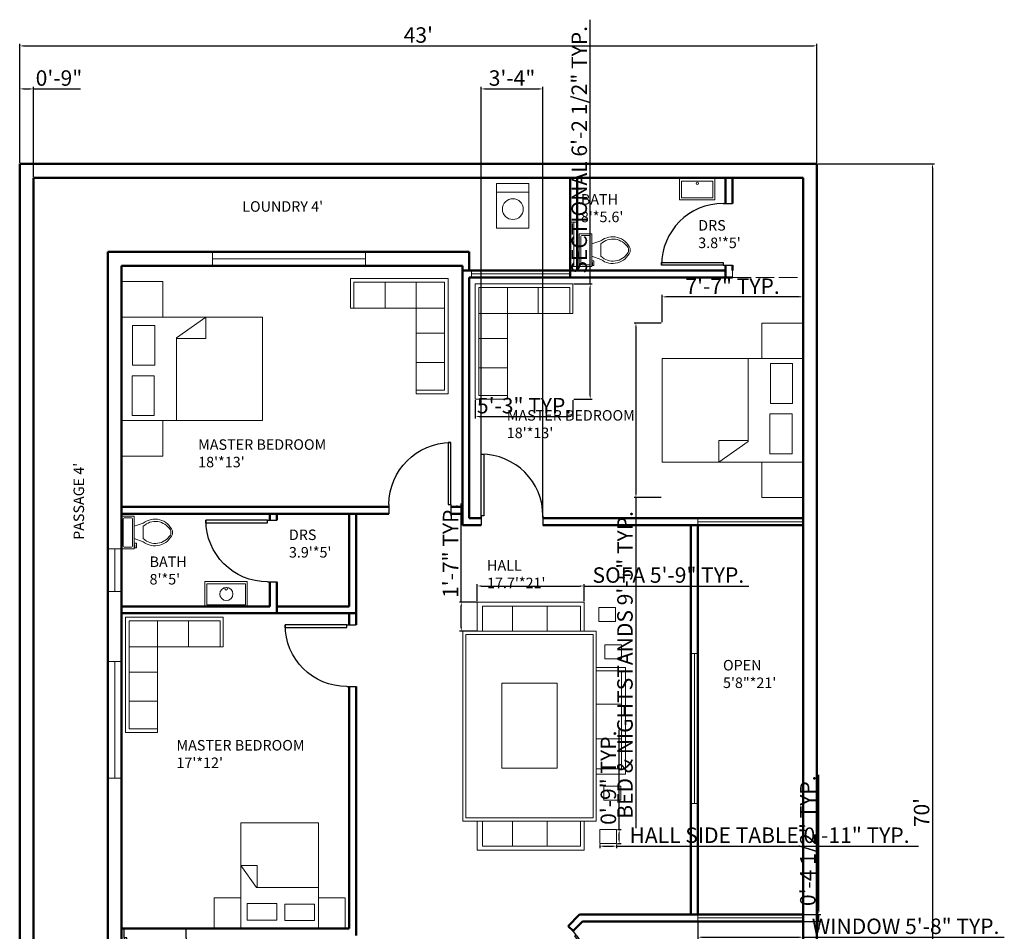
# Model space of a CAD drawing. Units: inches. Extents: x 2154 to 2791, y 2711 to 3705.
# Tile 2 of 2: x 2154 to 2791, y 3115 to 3705. Entities that reach past the tile are written whole.
import ezdxf

# ---------------------------------------------------------------- set-up
doc = ezdxf.new("R2010")
doc.units = ezdxf.units.IN
doc.linetypes.add('ACAD_ISO02W100', pattern=[15, 12, -3])
for name, color, linetype, lineweight in [('A-ANNO-DIMS', 2, 'Continuous', 18), ('A-AREA-IDEN', 104, 'Continuous', 25), ('A-DOOR', 4, 'Continuous', 25), ('A-EQPM', 8, 'Continuous', 18), ('A-FLOR-FIXT', 9, 'Continuous', 18), ('A-FURN', 8, 'Continuous', 18), ('A-WALL', 7, 'Continuous', 50), ('A-WALL-OVHD', 8, 'ACAD_ISO02W100', 18), ('WINDOW', 52, 'Continuous', 18)]:
    doc.layers.add(name, color=color, linetype=linetype, lineweight=lineweight)
doc.styles.get("Standard").update_dxf_attribs({"font": 'arial.ttf'})
doc.dimstyles.new('ISO-25', dxfattribs={"dimtxt": 10, "dimasz": 2.5, "dimexe": 1.25, "dimexo": 0.625, "dimtad": 1, "dimdec": 0, "dimlunit": 4, "dimtxsty": 'Standard', "dimcen": 2.5, "dimadec": 0, "dimazin": 0, "dimtfac": 1, "dimtdec": 0, "dimtmove": 0, "dimatfit": 3, "dimfxl": 1, "dimarcsym": 0})

# ---------------------------------------------------------------- blocks, each defined once
blk = doc.blocks.new('*U2')
for p, q in [((0, 0), (0, -6)), ((40, 0), (40, -6))]:
    blk.add_line(p, q)
blk.add_lwpolyline([(0, 0), (0, 40), (1.75, 40), (1.75, 0)], close=True)
blk.add_arc((0, 0), 40, 0, 90)
blk = doc.blocks.new('*U4')
for p, q in [((9.5, -6), (9.5, -2)), ((-10, -8.5), (-8, -8.5)), ((-10, -9.5), (-10, -8.5)), ((-7, -9.5), (-10, -9.5)), ((-8, -8.5), (-8, -8)), ((-7, -8), (-7, -9.5)), ((-4, -8), (-6, -14)), ((4, -8), (6, -14)), ((4, -14), (-4, -14))]:
    blk.add_line(p, q)
blk.add_lwpolyline([(10.5, -8), (10.5, 0), (-10.5, 0), (-10.5, -8)], close=True)
for points in [[(-9.5, -2), (-9.5, -6)], [(8.5, -1), (-8.5, -1)], [(-8.5, -7), (8.5, -7)]]:
    blk.add_lwpolyline(points)
for centre, radius, start, end in [((-8.62, -1.88), 0.884, 81.8699, 188.1301), ((-8.62, -6.12), 0.884, 171.8699, 278.1301), ((8.62, -1.88), 0.884, 351.8699, 98.1301), ((8.62, -6.12), 0.884, 261.8699, 8.1301), ((3.52, -21.58), 12.17, 141.46911, 247.97143), ((4.2, -21.82), 11.33, 136.36773, 238.94682), ((-3.52, -21.58), 12.17, 292.02843, 38.53071), ((-4.2, -21.82), 11.33, 301.05301, 43.63209), ((0, -27.88), 4, 245.73182, 294.26817), ((0, -29), 4, 254.86053, 285.13947)]:
    blk.add_arc(centre, radius, start, end)
blk = doc.blocks.new('*D5')
at = {"layer": 'A-ANNO-DIMS', "color": 0, "lineweight": -2, "transparency": 16777216}
for p, q in [((2153.51, 3612.02), (2153.51, 3689.01)), ((2156.01, 3687.76), (2667.01, 3687.76)), ((2669.51, 3612.02), (2669.51, 3689.01))]:
    blk.add_line(p, q, dxfattribs=at)
at = {"layer": 'A-ANNO-DIMS', "color": 0, "lineweight": 100, "transparency": 16777216}
for points in [[(2156.01, 3688.17), (2156.01, 3687.34), (2153.51, 3687.76)], [(2667.01, 3688.17), (2667.01, 3687.34), (2669.51, 3687.76)]]:
    blk.add_solid(points, dxfattribs=at)
at = {"layer": 'Defpoints', "color": 0, "lineweight": 100, "transparency": 16777216}
for p in [(2669.51, 3687.76), (2153.51, 3611.4), (2669.51, 3611.4)]:
    blk.add_point(p, dxfattribs=at)
at = {"layer": 'A-ANNO-DIMS', "color": 0, "transparency": 16777216, "insert": (2411.51, 3693.49), "char_height": 10, "attachment_point": 5}
blk.add_mtext("43'", dxfattribs=at)
blk = doc.blocks.new('*D6')
at = {"layer": 'A-ANNO-DIMS', "color": 0, "lineweight": -2, "transparency": 16777216}
for p, q in [((2670.13, 3611.4), (2745.54, 3611.4)), ((2744.29, 3608.9), (2744.29, 2773.9)), ((2670.13, 2771.4), (2745.54, 2771.4))]:
    blk.add_line(p, q, dxfattribs=at)
at = {"layer": 'A-ANNO-DIMS', "color": 0, "lineweight": 100, "transparency": 16777216}
for points in [[(2743.87, 3608.9), (2744.7, 3608.9), (2744.29, 3611.4)], [(2743.87, 2773.9), (2744.7, 2773.9), (2744.29, 2771.4)]]:
    blk.add_solid(points, dxfattribs=at)
at = {"layer": 'Defpoints', "color": 0, "lineweight": 100, "transparency": 16777216}
for p in [(2669.51, 3611.4), (2669.51, 2771.4), (2744.29, 2771.4)]:
    blk.add_point(p, dxfattribs=at)
at = {"layer": 'A-ANNO-DIMS', "color": 0, "transparency": 16777216, "insert": (2738.56, 3191.4), "char_height": 10, "attachment_point": 5, "rotation": 90}
blk.add_mtext("70'", dxfattribs=at)
blk = doc.blocks.new('BED-DOUBLE-NIGHTSTANDS')
for p, q in [((35.52, 76.7), (54.43, 90)), ((54.43, 90), (54.43, 76.12)), ((35.52, 23.03), (35.52, 76.7)), ((54.43, 76.12), (35.52, 76.12))]:
    blk.add_line(p, q)
for points in [[(0, 90), (26.57, 90), (26.57, 113.03), (0, 113.03)], [(0, 90), (91.17, 90), (91.17, 23.03), (0, 23.03)], [(7.11, 58.88), (21.43, 58.88), (21.43, 84.61), (7.11, 84.61)], [(6.72, 26.3), (21.05, 26.3), (21.05, 52.02), (6.72, 52.02)], [(0, 0), (26.57, 0), (26.57, 23.03), (0, 23.03)]]:
    blk.add_lwpolyline(points, close=True)
blk = doc.blocks.new('SEATING-L-SECTIONAL')
for p, q in [((63.18, 74.67), (0, 74.67)), ((0, 74.67), (0, 0)), ((40.71, 72.36), (40.71, 55.47)), ((63.18, 55.47), (63.18, 74.67)), ((63.18, 55.47), (54.76, 55.47)), ((20.77, 39.2), (2.41, 39.2)), ((20.77, 20.27), (2.41, 20.27)), ((20.77, 0), (20.77, 2.9)), ((0, 0), (20.77, 0))]:
    blk.add_line(p, q)
for points in [[(2.41, 72.36), (61.15, 72.36), (61.15, 55.47), (2.41, 55.47)], [(2.41, 72.36), (20.77, 72.36), (20.77, 2.4), (2.41, 2.4)]]:
    blk.add_lwpolyline(points, close=True)
blk = doc.blocks.new('SOFA-HALL-3SEAT')
for p, q in [((0, 0), (0, 18.94)), ((0, 18.94), (69.11, 18.94)), ((22.75, 16.33), (22.75, 0)), ((45.26, 16.33), (45.26, 0)), ((69.11, 18.94), (69.11, 0))]:
    blk.add_line(p, q)
blk.add_lwpolyline([(3.39, 0), (66.79, 0), (66.79, 16.33), (3.39, 16.33)], close=True)
blk = doc.blocks.new('BASIN-RECT')
for points in [[(27.46, 0), (0, 0), (0, 16.05), (27.46, 16.05)], [(1.33, 14.64), (26.38, 14.64), (26.38, 0.98), (1.33, 0.98)]]:
    blk.add_lwpolyline(points, close=True)
for centre, radius in [((13.96, 8), 4.26), ((13.84, 11.42), 0.841)]:
    blk.add_circle(centre, radius)
blk = doc.blocks.new('WINDOW-68IN')
blk.add_line((0, 2.25), (68, 2.25))
blk.add_lwpolyline([(0, 4.5), (68, 4.5), (68, 0), (0, 0)], close=True)
blk = doc.blocks.new('TABLE-END-RECT')
blk.add_lwpolyline([(0, 9.07), (10.91, 9.07), (10.91, 0), (0, 0)], close=True)
blk = doc.blocks.new('*D18')
at = {"layer": 'A-ANNO-DIMS', "color": 0, "lineweight": -2, "transparency": 16777216}
for p, q in [((2528.98, 3170.66), (2528.98, 3168.4)), ((2531.48, 3169.65), (2537.39, 3169.65)), ((2539.89, 3170.66), (2539.89, 3168.4)), ((2539.89, 3169.65), (2735.28, 3169.65))]:
    blk.add_line(p, q, dxfattribs=at)
at = {"layer": 'A-ANNO-DIMS', "color": 0, "lineweight": 100, "transparency": 16777216}
for points in [[(2531.48, 3170.07), (2531.48, 3169.24), (2528.98, 3169.65)], [(2537.39, 3170.07), (2537.39, 3169.24), (2539.89, 3169.65)]]:
    blk.add_solid(points, dxfattribs=at)
at = {"layer": 'Defpoints', "color": 0, "lineweight": 100, "transparency": 16777216}
for p in [(2528.98, 3171.29), (2539.89, 3171.29), (2539.89, 3169.65)]:
    blk.add_point(p, dxfattribs=at)
at = {"layer": 'A-ANNO-DIMS', "color": 0, "transparency": 16777216, "insert": (2638.84, 3175.45), "char_height": 10, "attachment_point": 5}
blk.add_mtext('HALL SIDE TABLE 0\'-11" TYP.', dxfattribs=at)
blk = doc.blocks.new('*D19')
at = {"layer": 'A-ANNO-DIMS', "color": 0, "lineweight": -2, "transparency": 16777216}
for p, q in [((2541.53, 3180.36), (2541.53, 3245.06)), ((2540.52, 3180.36), (2542.78, 3180.36)), ((2541.53, 3173.79), (2541.53, 3177.86)), ((2540.52, 3171.29), (2542.78, 3171.29))]:
    blk.add_line(p, q, dxfattribs=at)
at = {"layer": 'A-ANNO-DIMS', "color": 0, "lineweight": 100, "transparency": 16777216}
for points in [[(2541.11, 3177.86), (2541.95, 3177.86), (2541.53, 3180.36)], [(2541.11, 3173.79), (2541.95, 3173.79), (2541.53, 3171.29)]]:
    blk.add_solid(points, dxfattribs=at)
at = {"layer": 'Defpoints', "color": 0, "lineweight": 100, "transparency": 16777216}
for p in [(2539.89, 3180.36), (2541.53, 3180.36), (2539.89, 3171.29)]:
    blk.add_point(p, dxfattribs=at)
at = {"layer": 'A-ANNO-DIMS', "color": 0, "transparency": 16777216, "insert": (2535.8, 3213.96), "char_height": 10, "attachment_point": 5, "rotation": 90}
blk.add_mtext('0\'-9" TYP.', dxfattribs=at)
blk = doc.blocks.new('*D20')
at = {"layer": 'A-ANNO-DIMS', "color": 0, "lineweight": -2, "transparency": 16777216}
for p, q in [((2449.7, 3328.33), (2449.7, 3339.33)), ((2452.2, 3338.08), (2516.31, 3338.08)), ((2518.81, 3328.33), (2518.81, 3339.33)), ((2518.81, 3338.08), (2625.39, 3338.08))]:
    blk.add_line(p, q, dxfattribs=at)
at = {"layer": 'A-ANNO-DIMS', "color": 0, "lineweight": 100, "transparency": 16777216}
for points in [[(2452.2, 3338.49), (2452.2, 3337.66), (2449.7, 3338.08)], [(2516.31, 3338.49), (2516.31, 3337.66), (2518.81, 3338.08)]]:
    blk.add_solid(points, dxfattribs=at)
at = {"layer": 'Defpoints', "color": 0, "lineweight": 100, "transparency": 16777216}
for p in [(2518.81, 3338.08), (2449.7, 3327.71), (2518.81, 3327.71)]:
    blk.add_point(p, dxfattribs=at)
at = {"layer": 'A-ANNO-DIMS', "color": 0, "transparency": 16777216, "insert": (2573.35, 3343.87), "char_height": 10, "attachment_point": 5}
blk.add_mtext('SOFA 5\'-9" TYP.', dxfattribs=at)
blk = doc.blocks.new('*D21')
at = {"layer": 'A-ANNO-DIMS', "color": 0, "lineweight": -2, "transparency": 16777216}
for p, q in [((2439.33, 3327.71), (2439.33, 3391.47)), ((2449.07, 3327.71), (2438.08, 3327.71)), ((2439.33, 3311.26), (2439.33, 3325.21)), ((2449.07, 3308.76), (2438.08, 3308.76))]:
    blk.add_line(p, q, dxfattribs=at)
at = {"layer": 'A-ANNO-DIMS', "color": 0, "lineweight": 100, "transparency": 16777216}
for points in [[(2438.92, 3325.21), (2439.75, 3325.21), (2439.33, 3327.71)], [(2438.92, 3311.26), (2439.75, 3311.26), (2439.33, 3308.76)]]:
    blk.add_solid(points, dxfattribs=at)
at = {"layer": 'Defpoints', "color": 0, "lineweight": 100, "transparency": 16777216}
for p in [(2439.33, 3327.71), (2449.7, 3327.71), (2449.7, 3308.76)]:
    blk.add_point(p, dxfattribs=at)
at = {"layer": 'A-ANNO-DIMS', "color": 0, "transparency": 16777216, "insert": (2433.68, 3360.84), "char_height": 10, "attachment_point": 5, "rotation": 90}
blk.add_mtext('1\'-7" TYP.', dxfattribs=at)
blk = doc.blocks.new('*D24')
at = {"layer": 'A-ANNO-DIMS', "color": 0, "lineweight": -2, "transparency": 16777216}
for p, q in [((2568.71, 3508.32), (2551.13, 3508.32)), ((2552.38, 3505.82), (2552.38, 3397.79)), ((2568.71, 3395.29), (2551.13, 3395.29)), ((2552.38, 3395.29), (2552.38, 3181.22))]:
    blk.add_line(p, q, dxfattribs=at)
at = {"layer": 'A-ANNO-DIMS', "color": 0, "lineweight": 100, "transparency": 16777216}
for points in [[(2551.96, 3505.82), (2552.8, 3505.82), (2552.38, 3508.32)], [(2551.96, 3397.79), (2552.8, 3397.79), (2552.38, 3395.29)]]:
    blk.add_solid(points, dxfattribs=at)
at = {"layer": 'Defpoints', "color": 0, "lineweight": 100, "transparency": 16777216}
for p in [(2569.34, 3508.32), (2552.38, 3395.29), (2569.34, 3395.29)]:
    blk.add_point(p, dxfattribs=at)
at = {"layer": 'A-ANNO-DIMS', "color": 0, "transparency": 16777216, "insert": (2546.56, 3287), "char_height": 10, "attachment_point": 5, "rotation": 90}
blk.add_mtext('BED & NIGHTSTANDS 9\'-5" TYP.', dxfattribs=at)
blk = doc.blocks.new('*D25')
at = {"layer": 'A-ANNO-DIMS', "color": 0, "lineweight": -2, "transparency": 16777216}
for p, q in [((2569.34, 3508.94), (2569.34, 3526.52)), ((2658.01, 3525.27), (2571.84, 3525.27)), ((2660.51, 3508.94), (2660.51, 3526.52))]:
    blk.add_line(p, q, dxfattribs=at)
at = {"layer": 'A-ANNO-DIMS', "color": 0, "lineweight": 100, "transparency": 16777216}
for points in [[(2571.84, 3525.69), (2571.84, 3524.86), (2569.34, 3525.27)], [(2658.01, 3525.69), (2658.01, 3524.86), (2660.51, 3525.27)]]:
    blk.add_solid(points, dxfattribs=at)
at = {"layer": 'Defpoints', "color": 0, "lineweight": 100, "transparency": 16777216}
for p in [(2569.34, 3525.27), (2569.34, 3508.32), (2660.51, 3508.32)]:
    blk.add_point(p, dxfattribs=at)
at = {"layer": 'A-ANNO-DIMS', "color": 0, "transparency": 16777216, "insert": (2614.92, 3530.9), "char_height": 10, "attachment_point": 5}
blk.add_mtext('7\'-7" TYP.', dxfattribs=at)
blk = doc.blocks.new('*D26')
at = {"layer": 'A-ANNO-DIMS', "color": 0, "lineweight": -2, "transparency": 16777216}
for p, q in [((2522.77, 3533.69), (2522.77, 3704.71)), ((2512.19, 3533.69), (2524.02, 3533.69)), ((2522.77, 3461.51), (2522.77, 3531.19)), ((2512.19, 3459.01), (2524.02, 3459.01))]:
    blk.add_line(p, q, dxfattribs=at)
at = {"layer": 'A-ANNO-DIMS', "color": 0, "lineweight": 100, "transparency": 16777216}
for points in [[(2522.35, 3531.19), (2523.18, 3531.19), (2522.77, 3533.69)], [(2522.35, 3461.51), (2523.18, 3461.51), (2522.77, 3459.01)]]:
    blk.add_solid(points, dxfattribs=at)
at = {"layer": 'Defpoints', "color": 0, "lineweight": 100, "transparency": 16777216}
for p in [(2511.57, 3533.69), (2522.77, 3533.69), (2511.57, 3459.01)]:
    blk.add_point(p, dxfattribs=at)
at = {"layer": 'A-ANNO-DIMS', "color": 0, "transparency": 16777216, "insert": (2516.97, 3620.45), "char_height": 10, "attachment_point": 5, "rotation": 90}
blk.add_mtext('SECTIONAL 6\'-2 1/2" TYP.', dxfattribs=at)
blk = doc.blocks.new('*D27')
at = {"layer": 'A-ANNO-DIMS', "color": 0, "lineweight": -2, "transparency": 16777216}
for p, q in [((2448.38, 3458.39), (2448.38, 3446.56)), ((2511.57, 3458.39), (2511.57, 3446.56)), ((2450.88, 3447.81), (2509.07, 3447.81))]:
    blk.add_line(p, q, dxfattribs=at)
at = {"layer": 'A-ANNO-DIMS', "color": 0, "lineweight": 100, "transparency": 16777216}
for points in [[(2450.88, 3448.23), (2450.88, 3447.4), (2448.38, 3447.81)], [(2509.07, 3448.23), (2509.07, 3447.4), (2511.57, 3447.81)]]:
    blk.add_solid(points, dxfattribs=at)
at = {"layer": 'Defpoints', "color": 0, "lineweight": 100, "transparency": 16777216}
for p in [(2448.38, 3459.01), (2511.57, 3459.01), (2511.57, 3447.81)]:
    blk.add_point(p, dxfattribs=at)
at = {"layer": 'A-ANNO-DIMS', "color": 0, "transparency": 16777216, "insert": (2479.97, 3453.55), "char_height": 10, "attachment_point": 5}
blk.add_mtext('5\'-3" TYP.', dxfattribs=at)
blk = doc.blocks.new('*D30')
at = {"layer": 'A-ANNO-DIMS', "color": 0, "lineweight": -2, "transparency": 16777216}
for p, q in [((2592.51, 3120.27), (2592.51, 3109.45)), ((2660.51, 3120.27), (2660.51, 3109.45)), ((2595.01, 3110.7), (2658.01, 3110.7)), ((2660.51, 3110.7), (2790.8, 3110.7))]:
    blk.add_line(p, q, dxfattribs=at)
at = {"layer": 'A-ANNO-DIMS', "color": 0, "lineweight": 100, "transparency": 16777216}
for points in [[(2595.01, 3111.11), (2595.01, 3110.28), (2592.51, 3110.7)], [(2658.01, 3111.11), (2658.01, 3110.28), (2660.51, 3110.7)]]:
    blk.add_solid(points, dxfattribs=at)
at = {"layer": 'Defpoints', "color": 0, "lineweight": 100, "transparency": 16777216}
for p in [(2592.51, 3120.9), (2660.51, 3120.9), (2660.51, 3110.7)]:
    blk.add_point(p, dxfattribs=at)
at = {"layer": 'A-ANNO-DIMS', "color": 0, "transparency": 16777216, "insert": (2726.9, 3116.49), "char_height": 10, "attachment_point": 5}
blk.add_mtext('WINDOW 5\'-8" TYP.', dxfattribs=at)
blk = doc.blocks.new('*D31')
at = {"layer": 'A-ANNO-DIMS', "color": 0, "lineweight": -2, "transparency": 16777216}
for p, q in [((2670.71, 3127.9), (2670.71, 3215.9)), ((2661.13, 3125.4), (2671.96, 3125.4)), ((2670.71, 3120.9), (2670.71, 3125.4)), ((2661.13, 3120.9), (2671.96, 3120.9)), ((2670.71, 3118.4), (2670.71, 3115.9))]:
    blk.add_line(p, q, dxfattribs=at)
at = {"layer": 'A-ANNO-DIMS', "color": 0, "lineweight": 100, "transparency": 16777216}
for points in [[(2670.29, 3127.9), (2671.13, 3127.9), (2670.71, 3125.4)], [(2670.29, 3118.4), (2671.13, 3118.4), (2670.71, 3120.9)]]:
    blk.add_solid(points, dxfattribs=at)
at = {"layer": 'Defpoints', "color": 0, "lineweight": 100, "transparency": 16777216}
for p in [(2660.51, 3125.4), (2670.71, 3125.4), (2660.51, 3120.9)]:
    blk.add_point(p, dxfattribs=at)
at = {"layer": 'A-ANNO-DIMS', "color": 0, "transparency": 16777216, "insert": (2664.91, 3173.15), "char_height": 10, "attachment_point": 5, "rotation": 90}
blk.add_mtext('0\'-4 1/2" TYP.', dxfattribs=at)
blk = doc.blocks.new('*D37')
at = {"layer": 'A-ANNO-DIMS', "color": 0, "lineweight": -2, "transparency": 16777216}
for p, q in [((2452.18, 3382.52), (2452.18, 3661.15)), ((2454.68, 3659.9), (2489.68, 3659.9)), ((2492.18, 3382.52), (2492.18, 3661.15))]:
    blk.add_line(p, q, dxfattribs=at)
at = {"layer": 'A-ANNO-DIMS', "color": 0, "lineweight": 100, "transparency": 16777216}
for points in [[(2454.68, 3660.31), (2454.68, 3659.48), (2452.18, 3659.9)], [(2489.68, 3660.31), (2489.68, 3659.48), (2492.18, 3659.9)]]:
    blk.add_solid(points, dxfattribs=at)
at = {"layer": 'Defpoints', "color": 0, "lineweight": 100, "transparency": 16777216}
for p in [(2492.18, 3659.9), (2452.18, 3381.9), (2492.18, 3381.9)]:
    blk.add_point(p, dxfattribs=at)
at = {"layer": 'A-ANNO-DIMS', "color": 0, "transparency": 16777216, "insert": (2472.18, 3665.63), "char_height": 10, "attachment_point": 5}
blk.add_mtext('3\'-4"', dxfattribs=at)
blk = doc.blocks.new('*D38')
at = {"layer": 'A-ANNO-DIMS', "color": 0, "lineweight": -2, "transparency": 16777216}
for p, q in [((2153.51, 3612.02), (2153.51, 3661.15)), ((2156.01, 3659.9), (2160.01, 3659.9)), ((2162.51, 3603.02), (2162.51, 3661.15)), ((2162.51, 3659.9), (2192.84, 3659.9))]:
    blk.add_line(p, q, dxfattribs=at)
at = {"layer": 'A-ANNO-DIMS', "color": 0, "lineweight": 100, "transparency": 16777216}
for points in [[(2156.01, 3660.31), (2156.01, 3659.48), (2153.51, 3659.9)], [(2160.01, 3660.31), (2160.01, 3659.48), (2162.51, 3659.9)]]:
    blk.add_solid(points, dxfattribs=at)
at = {"layer": 'Defpoints', "color": 0, "lineweight": 100, "transparency": 16777216}
for p in [(2162.51, 3659.9), (2153.51, 3611.4), (2162.51, 3602.4)]:
    blk.add_point(p, dxfattribs=at)
at = {"layer": 'A-ANNO-DIMS', "color": 0, "transparency": 16777216, "insert": (2178.93, 3665.63), "char_height": 10, "attachment_point": 5}
blk.add_mtext('0\'-9"', dxfattribs=at)

msp = doc.modelspace()

# ---------------------------------------------------------------- linework, layer by layer
at = {"layer": 'A-EQPM'}
msp.add_line((2462.05, 3593.12), (2483.02, 3593.12), dxfattribs=at)
msp.add_lwpolyline([(2462.05, 3598.57), (2483.02, 3598.57), (2483.02, 3569.73), (2462.05, 3569.73)], close=True, dxfattribs=at)
msp.add_circle((2472.71, 3582.07), 6.74, dxfattribs=at)
at = {"layer": 'A-FLOR-FIXT'}
for points in [[(2603.37, 3602.4), (2580.65, 3602.4), (2580.65, 3587.99), (2603.37, 3587.99)], [(2581.95, 3600.21), (2602.24, 3600.21), (2602.24, 3589.29), (2581.95, 3589.29)]]:
    msp.add_lwpolyline(points, close=True, dxfattribs=at)
msp.add_circle((2592.09, 3598.78), 0.752, dxfattribs=at)
at = {"layer": 'A-FURN'}
for p, q in [((2367.69, 3518), (2367.69, 3537.2)), ((2367.69, 3537.2), (2430.88, 3537.2)), ((2430.88, 3537.2), (2430.88, 3462.53)), ((2390.17, 3534.89), (2390.17, 3518)), ((2369.72, 3518), (2367.69, 3518)), ((2369.72, 3518), (2369.72, 3518)), ((2410.1, 3501.73), (2428.47, 3501.73)), ((2410.1, 3482.8), (2428.47, 3482.8)), ((2410.1, 3462.53), (2410.1, 3465.43)), ((2430.88, 3462.53), (2410.1, 3462.53)), ((2306.68, 3143), (2296.72, 3157.17)), ((2296.72, 3157.17), (2307.11, 3157.17)), ((2307.11, 3157.17), (2307.11, 3143)), ((2346.88, 3143), (2306.68, 3143))]:
    msp.add_line(p, q, dxfattribs=at)
for points in [[(2428.47, 3534.89), (2369.72, 3534.89), (2369.72, 3518), (2428.47, 3518)], [(2428.47, 3534.89), (2410.1, 3534.89), (2410.1, 3464.93), (2428.47, 3464.93)], [(2440.3, 3308.76), (2526.61, 3308.76), (2526.61, 3185.91), (2440.3, 3185.91)], [(2442.3, 3306.76), (2524.61, 3306.76), (2524.61, 3187.91), (2442.3, 3187.91)], [(2465.53, 3275.08), (2501.39, 3275.08), (2501.39, 3220.11), (2465.53, 3220.11)], [(2296.72, 3116.4), (2296.72, 3184.69), (2346.88, 3184.69), (2346.88, 3116.4)], [(2296.72, 3116.4), (2296.72, 3136.3), (2279.46, 3136.3), (2279.46, 3116.4)], [(2364.13, 3116.4), (2364.13, 3136.3), (2346.88, 3136.3), (2346.88, 3116.4)], [(2320.02, 3121.72), (2320.02, 3132.45), (2300.76, 3132.45), (2300.76, 3121.72)], [(2344.43, 3121.43), (2344.43, 3132.16), (2325.16, 3132.16), (2325.16, 3121.43)]]:
    msp.add_lwpolyline(points, close=True, dxfattribs=at)
at = {"layer": 'A-WALL'}
for p, q in [((2153.51, 3611.4), (2669.51, 3611.4)), ((2153.51, 2771.4), (2153.51, 3611.4)), ((2669.51, 3611.4), (2669.51, 2771.4)), ((2162.51, 3602.4), (2660.51, 3602.4)), ((2162.51, 2780.4), (2162.51, 3602.4)), ((2162.51, 3602.4), (2162.51, 3554.4)), ((2509.91, 3537.88), (2509.91, 3602.4)), ((2514.41, 3547.98), (2514.41, 3602.4)), ((2610.41, 3602.4), (2610.41, 3585.75)), ((2660.51, 3602.4), (2614.91, 3602.4)), ((2614.91, 3602.4), (2614.91, 3585.75)), ((2660.51, 3602.4), (2660.51, 2780.4)), ((2210.51, 3554.4), (2440.01, 3554.4)), ((2210.51, 3554.4), (2210.51, 3161.24)), ((2210.51, 3554.4), (2444.51, 3554.4)), ((2444.51, 3554.4), (2444.51, 3542.38)), ((2219.51, 3545.4), (2440.01, 3545.4)), ((2219.51, 3545.4), (2219.51, 3161.24)), ((2219.51, 3545.4), (2219.51, 3389.4)), ((2440.01, 3545.4), (2440.01, 3542.38)), ((2440.01, 3545.4), (2440.01, 3542.38)), ((2514.41, 3542.38), (2514.41, 3547.98)), ((2610.41, 3545.75), (2610.41, 3537.9)), ((2614.91, 3545.75), (2614.91, 3542.4)), ((2440.01, 3377.4), (2440.01, 3542.38)), ((2440.01, 3542.38), (2517.91, 3542.38)), ((2444.51, 3381.9), (2444.51, 3537.88)), ((2444.51, 3537.88), (2517.91, 3537.88)), ((2610.41, 3537.88), (2509.91, 3537.88)), ((2610.41, 3542.38), (2514.41, 3542.38)), ((2610.41, 3537.88), (2614.91, 3537.88)), ((2660.51, 3537.9), (2660.51, 3381.9)), ((2219.51, 3389.4), (2392.53, 3389.4)), ((2219.51, 3384.9), (2392.53, 3384.9)), ((2219.51, 3384.9), (2219.51, 3324.9)), ((2315.51, 3380.74), (2315.51, 3384.9)), ((2320.01, 3380.74), (2320.01, 3384.9)), ((2366.81, 3324.9), (2366.81, 3384.9)), ((2371.31, 3320.4), (2371.31, 3384.9)), ((2432.53, 3389.4), (2435.51, 3389.4)), ((2432.53, 3384.9), (2435.51, 3384.9)), ((2435.51, 3389.4), (2440.01, 3389.4)), ((2435.51, 3384.9), (2440.01, 3384.9)), ((2452.18, 3381.9), (2444.51, 3381.9)), ((2660.51, 3381.9), (2492.18, 3381.9)), ((2452.18, 3377.4), (2440.01, 3377.4)), ((2660.51, 3377.4), (2492.18, 3377.4)), ((2588.01, 3377.4), (2588.01, 3125.4)), ((2592.51, 3377.4), (2592.51, 3125.4)), ((2315.51, 3324.9), (2315.51, 3340.74)), ((2320.01, 3320.4), (2320.01, 3340.74)), ((2219.51, 3324.9), (2315.51, 3324.9)), ((2219.51, 3320.4), (2320.01, 3320.4)), ((2219.51, 3320.4), (2371.31, 3320.4)), ((2219.51, 3320.4), (2363.51, 3320.4)), ((2320.01, 3324.9), (2366.81, 3324.9)), ((2320.01, 3320.4), (2371.31, 3320.4)), ((2363.51, 3320.4), (2366.81, 3320.4)), ((2366.81, 3320.4), (2366.81, 3312.97)), ((2371.31, 3320.4), (2371.31, 3312.97)), ((2366.81, 3272.97), (2366.81, 3116.4)), ((2371.31, 3272.97), (2371.31, 3111.9)), ((2219.51, 3116.4), (2219.51, 3172.99)), ((2210.51, 3161.24), (2210.51, 3045.59)), ((2515.82, 3125.4), (2508.51, 3117.96)), ((2660.51, 3125.4), (2515.82, 3125.4)), ((2222.81, 3116.4), (2219.51, 3116.4)), ((2219.51, 3116.4), (2219.51, 3061.2)), ((2366.81, 3116.4), (2222.81, 3116.4)), ((2508.51, 3117.96), (2511.72, 3114.81)), ((2517.7, 3120.9), (2511.72, 3114.81)), ((2660.51, 3120.9), (2517.7, 3120.9))]:
    msp.add_line(p, q, dxfattribs=at)
at = {"layer": 'A-WALL-OVHD'}
for p, q in [((2614.91, 3542.4), (2614.91, 3537.9)), ((2614.91, 3537.9), (2660.51, 3537.9))]:
    msp.add_line(p, q, dxfattribs=at)
at = {"layer": 'WINDOW'}
for p, q in [((2512.16, 3545.02), (2512.16, 3573.57)), ((2278.41, 3549.9), (2377.41, 3549.9)), ((2446.04, 3540.13), (2509.91, 3540.13)), ((2592.51, 3381.9), (2660.51, 3381.9)), ((2660.51, 3377.4), (2592.51, 3377.4)), ((2215.01, 3334.42), (2215.01, 3362.15)), ((2215.01, 3213.63), (2215.01, 3289.17)), ((2590.26, 3294.42), (2590.26, 3197.29)), ((2592.51, 3125.4), (2660.51, 3125.4)), ((2588.01, 3120.9), (2660.51, 3120.9))]:
    msp.add_line(p, q, dxfattribs=at)
for points in [[(2509.91, 3545.02), (2514.41, 3545.02), (2514.41, 3573.57), (2509.91, 3573.57)], [(2278.41, 3554.4), (2377.41, 3554.4), (2377.41, 3545.4), (2278.41, 3545.4)], [(2446.04, 3542.38), (2509.91, 3542.38), (2509.91, 3537.88), (2446.04, 3537.88)], [(2210.51, 3362.15), (2219.51, 3362.15), (2219.51, 3334.42), (2210.51, 3334.42)], [(2219.51, 3289.17), (2210.51, 3289.17), (2210.51, 3213.63), (2219.51, 3213.63)], [(2588.01, 3294.42), (2592.51, 3294.42), (2592.51, 3197.29), (2588.01, 3197.29)]]:
    msp.add_lwpolyline(points, close=True, dxfattribs=at)

# ---------------------------------------------------------------- block references
at = {"layer": 'A-DOOR', "rotation": 90}
msp.add_blockref('*U2', (2608.91, 3545.75), dxfattribs=at)
at = {"layer": 'A-DOOR', "xscale": -1}
msp.add_blockref('*U2', (2432.53, 3390.9), dxfattribs=at)
at = {"layer": 'A-DOOR'}
msp.add_blockref('*U2', (2452.18, 3383.4), dxfattribs=at)
at = {"layer": 'A-DOOR', "xscale": -1}
for p, rotation in [((2314.01, 3380.74), 90), ((2365.31, 3312.97), 90), ((2221.16, 3110.4), 180)]:
    msp.add_blockref('*U2', p, dxfattribs=dict(at, rotation=rotation))
at = {"layer": 'A-DOOR', "xscale": 0.5524960202192207, "yscale": 0.5524960202192207, "zscale": 0.5524960202192207, "rotation": 215.5609212162676}
msp.add_blockref('*U2', (2513.65, 3112.11), dxfattribs=at)
at = {"layer": 'A-FLOR-FIXT', "rotation": 90}
for p in [(2515.72, 3555.53), (2219.51, 3372.74)]:
    msp.add_blockref('*U4', p, dxfattribs=at)
at = {"layer": 'A-FLOR-FIXT'}
msp.add_blockref('BASIN-RECT', (2273.31, 3324.9), dxfattribs=at)
at = {"layer": 'A-FURN'}
for name, p in [('BED-DOUBLE-NIGHTSTANDS', (2219.51, 3422.13)), ('SEATING-L-SECTIONAL', (2448.38, 3459.01)), ('SOFA-HALL-3SEAT', (2449.7, 3308.76)), ('TABLE-END-RECT', (2528.34, 3315.06)), ('SEATING-L-SECTIONAL', (2222.04, 3243.16)), ('TABLE-END-RECT', (2532.22, 3291)), ('TABLE-END-RECT', (2531.61, 3199.46)), ('TABLE-END-RECT', (2528.98, 3171.29))]:
    msp.add_blockref(name, p, dxfattribs=at)
at = {"layer": 'A-FURN', "rotation": 180}
msp.add_blockref('BED-DOUBLE-NIGHTSTANDS', (2660.51, 3508.32), dxfattribs=at)
at = {"layer": 'A-FURN', "extrusion": (0, 0, -1), "zscale": -1}
for p, rotation in [((-2526.61, 3216.3), 89.99999999999918), ((-2449.7, 3185.91), 180)]:
    msp.add_blockref('SOFA-HALL-3SEAT', p, dxfattribs=dict(at, rotation=rotation))
at = {"layer": 'WINDOW'}
for p in [(2592.51, 3377.4), (2592.51, 3120.9)]:
    msp.add_blockref('WINDOW-68IN', p, dxfattribs=at)

# ---------------------------------------------------------------- texts
at = {"layer": 'A-AREA-IDEN', "attachment_point": 1}
for s, insert, char_height in [("BATH\\P8'*5.6'", (2516.71, 3591.77), 6.805), ("LOUNDRY 4'", (2297.54, 3587.19), 6.805), ("DRS\\P3.8'*5'", (2592.69, 3574.98), 6.805), ("MASTER BEDROOM\\P18'*13'", (2468.77, 3451.95), 6.8045), ("MASTER BEDROOM\\P18'*13'", (2269.04, 3433.05), 6.8045), ("DRS\\P3.9'*5'", (2327.76, 3374.65), 6.805), ("BATH\\P8'*5'", (2237.57, 3357.2), 6.805), ("HALL\\P17.7'*21'", (2455.99, 3354.81), 6.805), ('OPEN\\P5\'8"*21\'', (2608.72, 3290.19), 6.805), ("MASTER BEDROOM\\P17'*12'", (2254.99, 3238.38), 6.8045)]:
    msp.add_mtext_dynamic_manual_height_columns(s, width=177.5689, gutter_width=34.02, heights=[0], dxfattribs=dict(at, insert=insert, char_height=char_height))
at = {"layer": 'A-AREA-IDEN', "insert": (2188.37, 3367.94), "char_height": 6.805, "attachment_point": 1, "rotation": 90}
msp.add_mtext_dynamic_manual_height_columns("PASSAGE 4'", width=177.5689, gutter_width=34.02, heights=[0], dxfattribs=at)

# ---------------------------------------------------------------- dimensions: what is measured, and where the dimension line sits
at = {"layer": 'A-ANNO-DIMS'}
for base, p1, p2, angle, text, picture, middle in [((2522.77, 3533.69), (2511.57, 3459.01), (2511.57, 3533.69), 90, 'SECTIONAL <> TYP.', '*D26', (2516.97, 3620.45)), ((2569.34, 3525.27), (2660.51, 3508.32), (2569.34, 3508.32), 180, '<> TYP.', '*D25', (2614.92, 3530.9)), ((2552.38, 3395.29), (2569.34, 3508.32), (2569.34, 3395.29), 270, 'BED & NIGHTSTANDS <> TYP.', '*D24', (2546.56, 3287)), ((2439.3325, 3327.7079), (2449.6998, 3308.7639), (2449.6998, 3327.7079), 90, '<> TYP.', '*D21', (2433.6837, 3360.8397)), ((2541.53, 3180.36), (2539.89, 3171.29), (2539.89, 3180.36), 90, '<> TYP.', '*D19', (2535.8, 3213.96)), ((2670.71, 3125.4), (2660.51, 3120.9), (2660.51, 3125.4), 90, '<> TYP.', '*D31', (2664.91, 3173.15))]:
    dim = msp.add_linear_dim(base=base, p1=p1, p2=p2, angle=angle, text=text, dimstyle='ISO-25', override={"dimdec": 1, "dimlfac": 1, "dimrnd": 0, "dimzin": 1, "dimdsep": 46, "dimlunit": 4, "dimfrac": 2}, dxfattribs=at)
    dim.commit()
    dim.dimension.update_dxf_attribs({"geometry": picture, "text_midpoint": middle})
for base, p1, p2, override, picture, middle in [((2669.51, 3687.76), (2153.51, 3611.4), (2669.51, 3611.4), {"dimclrd": 0, "dimclre": 0, "dimclrt": 0}, '*D5', (2411.51, 3693.49)), ((2162.51, 3659.9), (2153.51, 3611.4), (2162.51, 3602.4), {"dimdec": 1, "dimlfac": 1, "dimrnd": 0, "dimzin": 1, "dimdsep": 46, "dimlunit": 4, "dimfrac": 2}, '*D38', (2178.93, 3665.63)), ((2492.18, 3659.9), (2452.18, 3381.9), (2492.18, 3381.9), {"dimdec": 1, "dimlfac": 1, "dimrnd": 0, "dimzin": 1, "dimdsep": 46, "dimlunit": 4, "dimfrac": 2}, '*D37', (2472.18, 3665.63))]:
    dim = msp.add_linear_dim(base=base, p1=p1, p2=p2, dimstyle='ISO-25', override=override, dxfattribs=at)
    dim.commit()
    dim.dimension.update_dxf_attribs({"geometry": picture, "text_midpoint": middle})
dim = msp.add_linear_dim(base=(2744.29, 2771.4), p1=(2669.51, 3611.4), p2=(2669.51, 2771.4), angle=90, dimstyle='ISO-25', override={"dimclrd": 0, "dimclre": 0, "dimclrt": 0}, dxfattribs=at)
dim.commit()
dim.dimension.update_dxf_attribs({"geometry": '*D6', "text_midpoint": (2738.56, 3191.4)})
for base, p1, p2, text, picture, middle in [((2511.57, 3447.81), (2448.38, 3459.01), (2511.57, 3459.01), '<> TYP.', '*D27', (2479.97, 3453.55)), ((2518.81, 3338.08), (2449.7, 3327.71), (2518.81, 3327.71), 'SOFA <> TYP.', '*D20', (2573.35, 3343.87)), ((2539.89, 3169.65), (2528.98, 3171.29), (2539.89, 3171.29), 'HALL SIDE TABLE <> TYP.', '*D18', (2638.84, 3175.45)), ((2660.51, 3110.7), (2592.51, 3120.9), (2660.51, 3120.9), 'WINDOW <> TYP.', '*D30', (2726.9, 3116.49))]:
    dim = msp.add_linear_dim(base=base, p1=p1, p2=p2, text=text, dimstyle='ISO-25', override={"dimdec": 1, "dimlfac": 1, "dimrnd": 0, "dimzin": 1, "dimdsep": 46, "dimlunit": 4, "dimfrac": 2}, dxfattribs=at)
    dim.commit()
    dim.dimension.update_dxf_attribs({"geometry": picture, "text_midpoint": middle})

doc.saveas('drawing.dxf')
